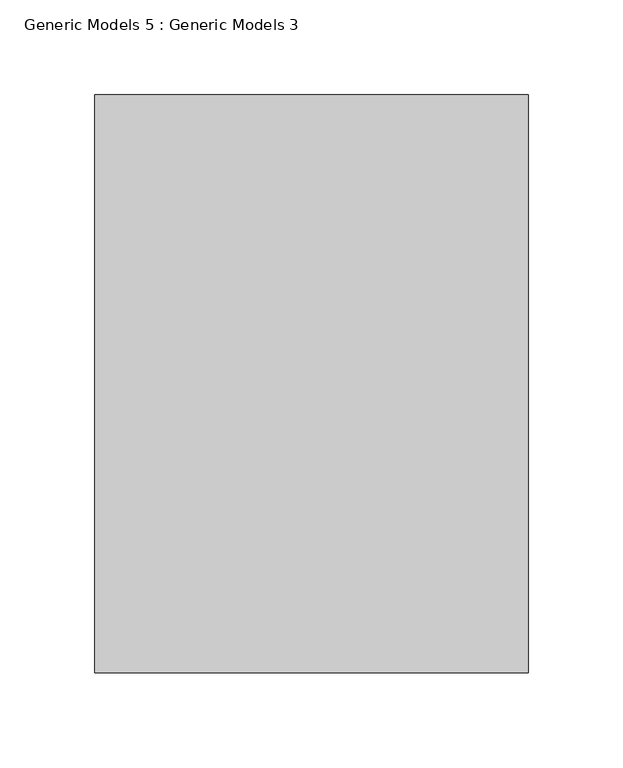
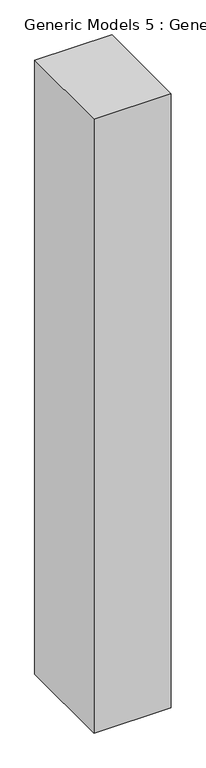
"""IFC4 building model written with IfcOpenShell, lengths in millimetres: proxy geometry, Generic Models 5 : Generic Models 3."""

from ifc_helpers import new_model, si_unit, frame, origin, place, context, project, spatial, polyline, outline, extrude, source, transform, mapped, element, save


def generic_models_5_generic_models_3_4887dcf5(model_context):
    return source(origin(), model_context, "Body", "SweptSolid", [
        extrude(outline(polyline([(-19710.968705, -5256.7027976), (-19482.368705, -5256.7027976), (-19482.368705, -5561.5027976), (-19710.968705, -5561.5027976), (-19710.968705, -5256.7027976)])), frame((0.0, 0.0, 457.2), z_axis=(0.0, 0.0, 1.0), x_axis=(1.0, 0.0, 0.0)), (0.0, 0.0, 1.0), 1922.2594115),
    ])


if __name__ == "__main__":
    model = new_model("IFC4")
    model_context = context("Model", 3, world=origin())
    ifc_project = project(units=[si_unit("LENGTHUNIT", "METRE", prefix="MILLI")], contexts=[model_context])
    site = spatial("IfcSite", under=ifc_project)
    building = spatial("IfcBuilding", under=site)
    placement = place(None, origin())
    generic_models_5_generic_models_3_shape = generic_models_5_generic_models_3_4887dcf5(model_context)
    element("IfcBuildingElementProxy", 1, Name="Generic Models 5 : Generic Models 3", ObjectType="Generic Models 5 : Generic Models 3", at=placement, inside=building, context=model_context, shape_type="MappedRepresentation", body=[
        mapped(generic_models_5_generic_models_3_shape, transform((0.0, 0.0, 0.0), x_axis=(1.0, 0.0, 0.0), y_axis=(0.0, 1.0, 0.0), z_axis=(0.0, 0.0, 1.0))),
    ])
    save(model, "model.ifc")
